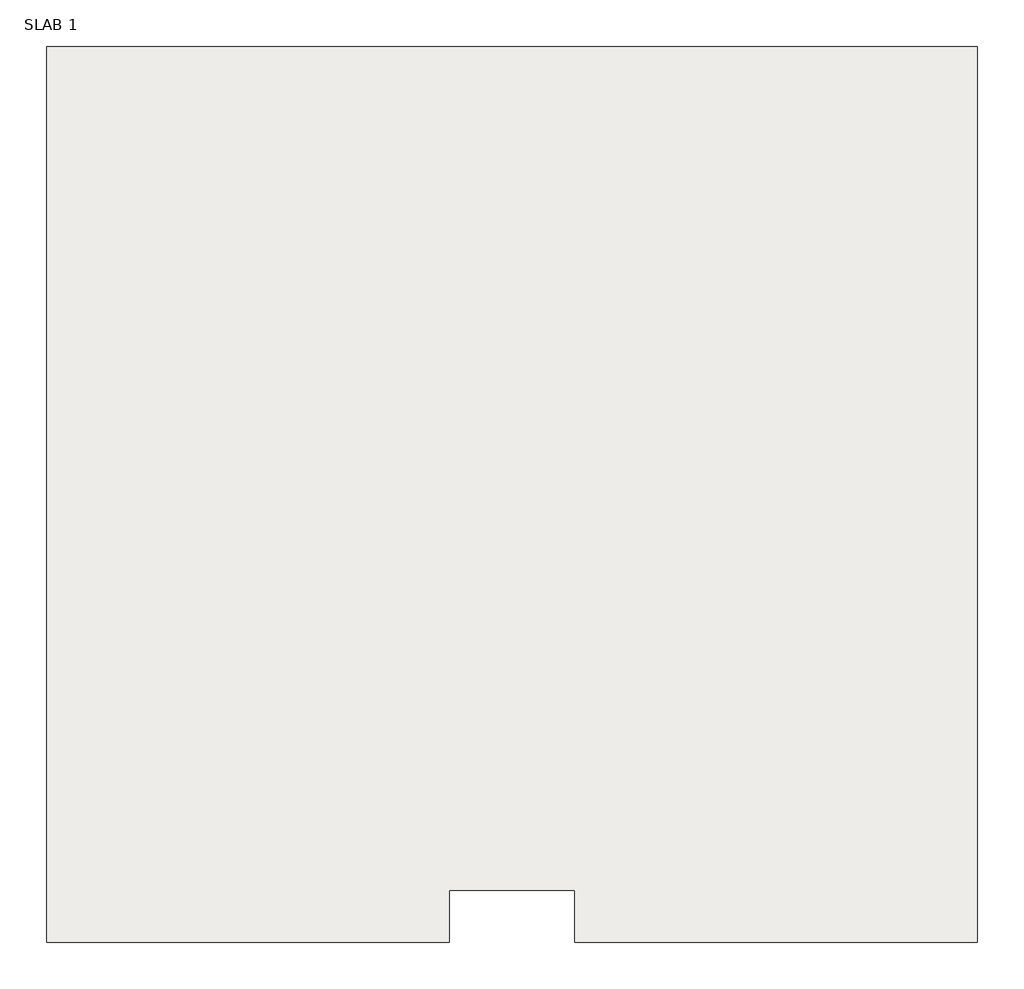
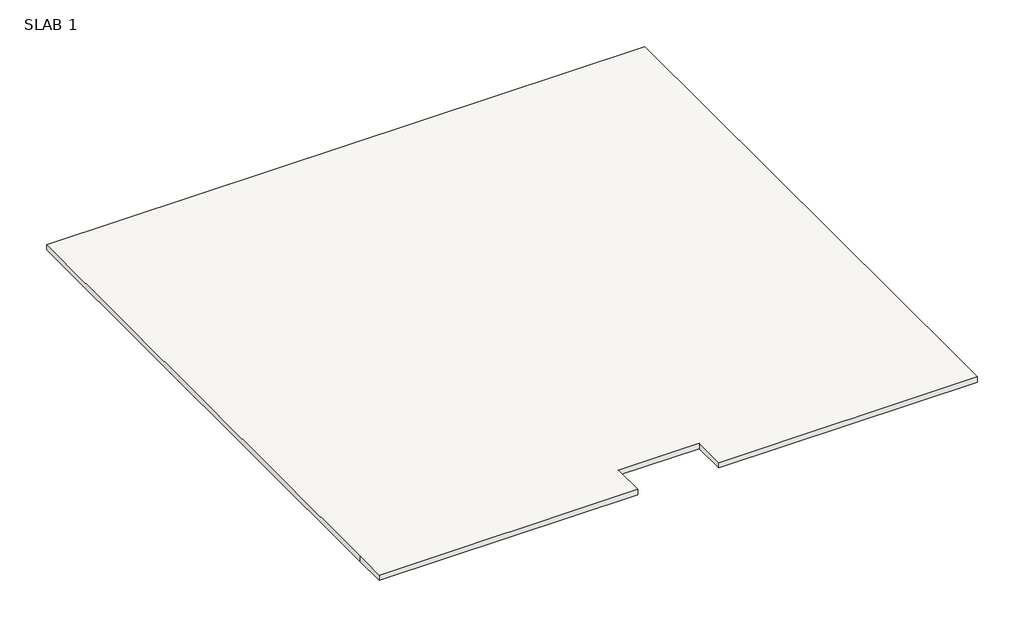
# One storey: 2 roofs.
"""IFC4 building model written with IfcOpenShell, lengths in millimetres."""

from ifc_helpers import new_model, si_unit, frame, origin, place, context, project, spatial, polyline, outline, extrude, element, save

model = new_model("IFC4")

# Units and contexts
model_context = context("Model", 3, world=origin())
ifc_project = project(units=[si_unit("LENGTHUNIT", "METRE", prefix="MILLI")], contexts=[model_context])

# Site, building, storey
site = spatial("IfcSite", under=ifc_project)
building = spatial("IfcBuilding", under=site)
storey = spatial("IfcBuildingStorey", under=building, Name="SLAB 1", Elevation=3048.0)

# Roofs
placement = place(None, origin())
element("IfcRoof", 1, ObjectType="ROOFING 6\"", at=placement, inside=storey, context=model_context, shape_type="SweptSolid", body=[
    extrude(outline(polyline([(-3159.4137331, -7822.4593836), (-5369.2137331, -7822.4593836), (-5369.2137331, -8736.8593836), (-12430.4137331, -8736.8593836), (-12430.4137331, -7822.4593836), (-12430.4137331, 6987.3281164), (3901.7862669, 6987.3281164), (3901.7862669, -7822.4593836), (3901.7862669, -8736.8593836), (-3159.4137331, -8736.8593836), (-3159.4137331, -7822.4593836)])), frame((0.0, 0.0, 3048.0), z_axis=(0.0, 0.0, 1.0), x_axis=(1.0, 0.0, 0.0)), (0.0, 0.0, 1.0), 152.4),
])
element("IfcRoof", 2, ObjectType="ROOFING 6\"", at=placement, inside=storey, context=model_context, shape_type="SweptSolid", body=[
    extrude(outline(polyline([(-3159.4137331, -7822.4593836), (-5369.2137331, -7822.4593836), (-5369.2137331, -8736.8593836), (-12430.4137331, -8736.8593836), (-12430.4137331, -7822.4593836), (-12430.4137331, 6987.3281164), (3901.7862669, 6987.3281164), (3901.7862669, -7822.4593836), (3901.7862669, -8736.8593836), (-3159.4137331, -8736.8593836), (-3159.4137331, -7822.4593836)])), frame((0.0, 0.0, 3048.0), z_axis=(0.0, 0.0, 1.0), x_axis=(1.0, 0.0, 0.0)), (0.0, 0.0, 1.0), 152.4),
])

save(model, "model.ifc")

# Revit data of these elements
# Type "ROOFING 6\""
#   Assembly Code = "B1020"
#   Layers, outside or top first: 0' - 6" no material (function 1)
# Element 1 (IfcRoof, "ROOFING 6\"")
#   built-in parameter 1001705 = 10.5 (stored number, unit not read)
#   built-in parameter 1001710 = 33615
#   Phase Created = New Construction
#   Materials on its faces: "Default Roof"
# Element 2 (IfcRoof, "ROOFING 6\"")
#   built-in parameter 1001705 = 10.5 (stored number, unit not read)
#   built-in parameter 1001710 = 33615
#   Phase Created = New Construction
#   Materials on its faces: "Default Roof", "Clad - White"
# Materials
#   "Default Roof": colour RGB 88 101 114, transparency 0, Cost = 0
#   "Clad - White": class "Wood", colour RGB 242 242 238, transparency 0, Cost = 0
